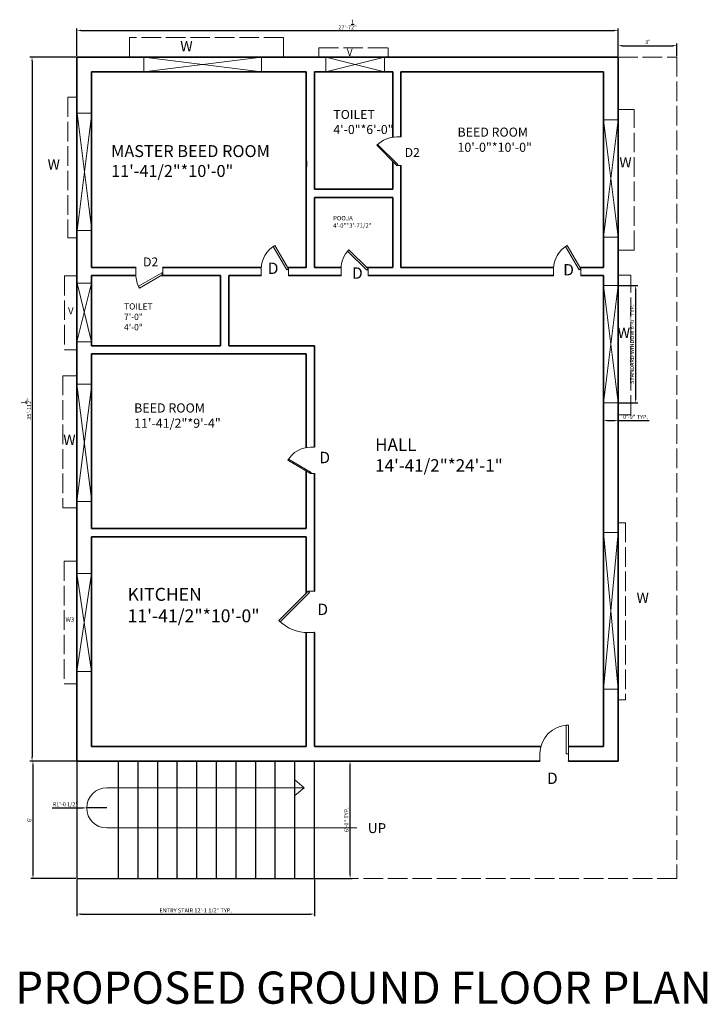
# Model space of a CAD drawing. Units: millimetres. Extents: x 3312 to 4717, y 967 to 1587.
# Tile 1 of 2: x 3312 to 3733, y 967 to 1571. Entities that reach past the tile are written whole.
import ezdxf

# ---------------------------------------------------------------- set-up
doc = ezdxf.new("R2010")
doc.units = ezdxf.units.MM
doc.linetypes.add('ACAD_ISO02W100', pattern=[15, 12, -3])
for name, color, linetype, lineweight, true_color in [('A-ANNO-DIMS', 116, 'Continuous', 18, 0x136734), ('A-ANNO-IDEN', 116, 'Continuous', 18, 0x136734), ('A-ANNO-SYMB', 219, 'Continuous', 18, 0x642165), ('A-ANNO-TEXT', 55, 'Continuous', 18, 0x999b37), ('A-ANNO-TITL', 116, 'Continuous', 35, 0x136734), ('A-AREA-IDEN', 244, 'Continuous', 18, 0x991b1e), ('A-GLAZ', 219, 'Continuous', 18, 0x642165), ('A-GLAZ-OVHD', 67, 'ACAD_ISO02W100', 13, 0x727430), ('C-PROP', 67, 'ACAD_ISO02W100', 18, 0x727430)]:
    doc.layers.add(name, color=color, linetype=linetype, lineweight=lineweight, true_color=true_color)
for name, color, linetype, lineweight in [('A-DOOR', 4, 'Continuous', 18), ('A-FLOR-STRS', 7, 'Continuous', 25), ('A-WALL', 7, 'Continuous', 35)]:
    doc.layers.add(name, color=color, linetype=linetype, lineweight=lineweight)
doc.styles.get("Standard").update_dxf_attribs({"font": 'arial.ttf'})
doc.dimstyles.new('ISO-25', dxfattribs={"dimtxt": 2.5, "dimasz": 2.5, "dimexe": 1.25, "dimexo": 0.625, "dimtad": 1, "dimdec": 3, "dimlunit": 4, "dimtxsty": 'Standard', "dimcen": 2.5, "dimadec": 0, "dimazin": 0, "dimtfac": 1, "dimtdec": 3, "dimtmove": 0, "dimatfit": 3, "dimfxl": 1, "dimarcsym": 0})

# ---------------------------------------------------------------- blocks, each defined once
blk = doc.blocks.new('*U3')
for p, q in [((-24, 0), (-24, 6)), ((0, 0), (0, 6))]:
    blk.add_line(p, q)
blk.add_lwpolyline([(0, 0), (-20.78, -12), (-21.66, -10.48), (-0.88, 1.52)], close=True)
blk.add_arc((0, 0), 24, 180, 210)
blk = doc.blocks.new('*U4')
for p, q in [((-24, 0), (-24, -6)), ((0, 0), (0, -6))]:
    blk.add_line(p, q)
blk.add_lwpolyline([(0, 0), (-12, 20.78), (-13.52, 19.91), (-1.52, -0.88)], close=True)
blk.add_arc((0, 0), 24, 120, 180)
blk = doc.blocks.new('*U5')
for p, q in [((0, 0), (0, -6)), ((40, 0), (40, -6))]:
    blk.add_line(p, q)
blk.add_lwpolyline([(0, 0), (28.3, 28.3), (29.5, 27), (1.2, -1.2)], close=True)
blk.add_arc((0, 0), 40, 0, 45)
blk = doc.blocks.new('*U7')
for p, q in [((0, 0), (0, -6)), ((40, 0), (40, -6))]:
    blk.add_line(p, q)
blk.add_lwpolyline([(0, 0), (20, 34.6), (21.5, 33.8), (1.5, -0.9)], close=True)
blk.add_arc((0, 0), 40, 0, 60)
blk = doc.blocks.new('*U6')
for p, q in [((0, 0), (0, 6)), ((40, 0), (40, 6))]:
    blk.add_line(p, q)
blk.add_lwpolyline([(0, 0), (28.28, -28.28), (29.52, -27.05), (1.24, 1.24)], close=True)
blk.add_arc((0, 0), 40, 315, 360)
blk = doc.blocks.new('*U2')
for p, q in [((0, 0), (0, -6)), ((24, 0), (24, -6))]:
    blk.add_line(p, q)
blk.add_lwpolyline([(0, 0), (0, 24), (1.75, 24), (1.75, 0)], close=True)
blk.add_arc((0, 0), 24, 0, 90)
blk = doc.blocks.new('*U8')
for p, q in [((-24, 0), (-24, -6)), ((0, 0), (0, -6))]:
    blk.add_line(p, q)
blk.add_lwpolyline([(0, 0), (-16.97, 16.97), (-18.21, 15.73), (-1.24, -1.24)], close=True)
blk.add_arc((0, 0), 24, 135, 180)
blk = doc.blocks.new('*D9')
at = {"layer": 'A-ANNO-DIMS', "color": 0, "lineweight": -2, "transparency": 16777216}
for p, q in [((3678.84, 1548.26), (3678.84, 1555.85)), ((3681.34, 1554.6), (3712.34, 1554.6)), ((3714.84, 1548.26), (3714.84, 1555.85))]:
    blk.add_line(p, q, dxfattribs=at)
at = {"layer": 'A-ANNO-DIMS', "color": 0, "lineweight": 5, "transparency": 16777216}
for points in [[(3681.34, 1555.02), (3681.34, 1554.18), (3678.84, 1554.6)], [(3712.34, 1555.02), (3712.34, 1554.18), (3714.84, 1554.6)]]:
    blk.add_solid(points, dxfattribs=at)
at = {"layer": 'Defpoints', "color": 0, "lineweight": 5, "transparency": 16777216}
for p in [(3714.84, 1554.6), (3678.84, 1547.64), (3714.84, 1547.64)]:
    blk.add_point(p, dxfattribs=at)
at = {"layer": 'A-ANNO-DIMS', "color": 0, "transparency": 16777216, "insert": (3696.84, 1556.5), "char_height": 2.5, "attachment_point": 5}
blk.add_mtext("3'", dxfattribs=at)
blk = doc.blocks.new('*D10')
at = {"layer": 'A-ANNO-DIMS', "color": 0, "lineweight": -2, "transparency": 16777216}
for p, q in [((3347.34, 1548.26), (3347.34, 1565.23)), ((3349.84, 1563.98), (3676.34, 1563.98)), ((3678.84, 1548.26), (3678.84, 1565.23))]:
    blk.add_line(p, q, dxfattribs=at)
at = {"layer": 'A-ANNO-DIMS', "color": 0, "lineweight": 5, "transparency": 16777216}
for points in [[(3349.84, 1564.4), (3349.84, 1563.57), (3347.34, 1563.98)], [(3676.34, 1564.4), (3676.34, 1563.57), (3678.84, 1563.98)]]:
    blk.add_solid(points, dxfattribs=at)
at = {"layer": 'Defpoints', "color": 0, "lineweight": 5, "transparency": 16777216}
for p in [(3678.84, 1563.98), (3347.34, 1547.64), (3678.84, 1547.64)]:
    blk.add_point(p, dxfattribs=at)
at = {"layer": 'A-ANNO-DIMS', "color": 0, "transparency": 16777216, "insert": (3513.09, 1567.54), "char_height": 2.5, "attachment_point": 5}
blk.add_mtext('27\'-7{\\H1x;\\S1/2;}"', dxfattribs=at)
blk = doc.blocks.new('*D11')
at = {"layer": 'A-ANNO-DIMS', "color": 0, "lineweight": -2, "transparency": 16777216}
for p, q in [((3346.71, 1547.64), (3318.6, 1547.64)), ((3319.85, 1545.14), (3319.85, 1118.64)), ((3346.71, 1116.14), (3318.6, 1116.14))]:
    blk.add_line(p, q, dxfattribs=at)
at = {"layer": 'A-ANNO-DIMS', "color": 0, "lineweight": 5, "transparency": 16777216}
for points in [[(3319.43, 1545.14), (3320.27, 1545.14), (3319.85, 1547.64)], [(3319.43, 1118.64), (3320.27, 1118.64), (3319.85, 1116.14)]]:
    blk.add_solid(points, dxfattribs=at)
at = {"layer": 'Defpoints', "color": 0, "lineweight": 5, "transparency": 16777216}
for p in [(3347.34, 1547.64), (3319.85, 1116.14), (3347.34, 1116.14)]:
    blk.add_point(p, dxfattribs=at)
at = {"layer": 'A-ANNO-DIMS', "color": 0, "transparency": 16777216, "insert": (3316.27, 1331.89), "char_height": 2.5, "attachment_point": 5, "rotation": 90}
blk.add_mtext('35\'-11{\\H1x;\\S1/2;}"', dxfattribs=at)
blk = doc.blocks.new('*D12')
at = {"layer": 'A-ANNO-DIMS', "color": 0, "lineweight": -2, "transparency": 16777216}
for p, q in [((3346.71, 1116.14), (3319.16, 1116.14)), ((3320.41, 1113.64), (3320.41, 1046.64)), ((3346.71, 1044.14), (3319.16, 1044.14))]:
    blk.add_line(p, q, dxfattribs=at)
at = {"layer": 'A-ANNO-DIMS', "color": 0, "lineweight": 5, "transparency": 16777216}
for points in [[(3320, 1113.64), (3320.83, 1113.64), (3320.41, 1116.14)], [(3320, 1046.64), (3320.83, 1046.64), (3320.41, 1044.14)]]:
    blk.add_solid(points, dxfattribs=at)
at = {"layer": 'Defpoints', "color": 0, "lineweight": 5, "transparency": 16777216}
for p in [(3347.34, 1116.14), (3320.41, 1044.14), (3347.34, 1044.14)]:
    blk.add_point(p, dxfattribs=at)
at = {"layer": 'A-ANNO-DIMS', "color": 0, "transparency": 16777216, "insert": (3318.51, 1080.14), "char_height": 2.5, "attachment_point": 5, "rotation": 90}
blk.add_mtext("6'", dxfattribs=at)
blk = doc.blocks.new('WIN-STANDARD')
for p, q in [((0, 72), (0, 0)), ((0, 0), (9, 72)), ((9, 72), (0, 72)), ((0, 72), (9, 0)), ((9, 0), (9, 72)), ((0, 0), (9, 0)), ((9, 0), (0, 0))]:
    blk.add_line(p, q)
blk = doc.blocks.new('GLAZ-NARROW')
for p, q in [((9, 35.99), (0.01, 35.99)), ((0.01, 35.99), (0.01, 0)), ((0.01, 0), (9, 35.99)), ((0.07, 35.99), (9, 0)), ((9, 0), (9, 35.99)), ((0, 0), (9, 0))]:
    blk.add_line(p, q)
blk = doc.blocks.new('STAIR-ENTRY-FLIGHT')
for p, q in [((0, 72), (0, 0)), ((145.5, 72), (0, 72)), ((25.5, 0), (25.5, 72)), ((37.5, 0), (37.5, 72)), ((49.5, 0), (49.5, 72)), ((61.5, 0), (61.5, 72)), ((73.5, 0), (73.5, 72)), ((85.5, 0), (85.5, 72)), ((97.5, 0), (97.5, 72)), ((109.5, 0), (109.5, 72)), ((121.5, 0), (121.5, 72)), ((133.5, 0), (133.5, 72)), ((145.5, 0), (145.5, 72)), ((0, 0), (145.5, 0))]:
    blk.add_line(p, q)
blk = doc.blocks.new('*D26')
at = {"layer": 'A-ANNO-DIMS', "color": 0, "lineweight": -2, "transparency": 16777216}
for p, q in [((3679.46, 1407.62), (3690.89, 1407.62)), ((3689.64, 1338.12), (3689.64, 1405.12)), ((3679.46, 1335.62), (3690.89, 1335.62))]:
    blk.add_line(p, q, dxfattribs=at)
at = {"layer": 'A-ANNO-DIMS', "color": 0, "lineweight": 5, "transparency": 16777216}
for points in [[(3689.22, 1405.12), (3690.05, 1405.12), (3689.64, 1407.62)], [(3689.22, 1338.12), (3690.05, 1338.12), (3689.64, 1335.62)]]:
    blk.add_solid(points, dxfattribs=at)
at = {"layer": 'Defpoints', "color": 0, "lineweight": 5, "transparency": 16777216}
for p in [(3678.84, 1407.62), (3689.64, 1407.62), (3678.84, 1335.62)]:
    blk.add_point(p, dxfattribs=at)
at = {"layer": 'A-ANNO-DIMS', "color": 0, "transparency": 16777216, "insert": (3687.72, 1371.62), "char_height": 2.5, "attachment_point": 5, "rotation": 90}
blk.add_mtext('STANDARD WINDOW 6\'-0" TYP.', dxfattribs=at)
blk = doc.blocks.new('*D27')
at = {"layer": 'A-ANNO-DIMS', "color": 0, "lineweight": -2, "transparency": 16777216}
for p, q in [((3669.84, 1335), (3669.84, 1323.57)), ((3678.84, 1335), (3678.84, 1323.57)), ((3672.34, 1324.82), (3676.34, 1324.82)), ((3678.84, 1324.82), (3697.82, 1324.82))]:
    blk.add_line(p, q, dxfattribs=at)
at = {"layer": 'A-ANNO-DIMS', "color": 0, "lineweight": 5, "transparency": 16777216}
for points in [[(3672.34, 1325.24), (3672.34, 1324.4), (3669.84, 1324.82)], [(3676.34, 1325.24), (3676.34, 1324.4), (3678.84, 1324.82)]]:
    blk.add_solid(points, dxfattribs=at)
at = {"layer": 'Defpoints', "color": 0, "lineweight": 5, "transparency": 16777216}
for p in [(3669.84, 1335.62), (3678.84, 1335.62), (3678.84, 1324.82)]:
    blk.add_point(p, dxfattribs=at)
at = {"layer": 'A-ANNO-DIMS', "color": 0, "transparency": 16777216, "insert": (3689.58, 1326.72), "char_height": 2.5, "attachment_point": 5}
blk.add_mtext('0\'-9" TYP.', dxfattribs=at)
blk = doc.blocks.new('*D32')
at = {"layer": 'A-ANNO-DIMS', "color": 0, "lineweight": -2, "transparency": 16777216}
for p, q in [((3347.34, 1043.51), (3347.34, 1021.06)), ((3492.84, 1043.51), (3492.84, 1021.06)), ((3349.84, 1022.31), (3490.34, 1022.31))]:
    blk.add_line(p, q, dxfattribs=at)
at = {"layer": 'A-ANNO-DIMS', "color": 0, "lineweight": 5, "transparency": 16777216}
for points in [[(3349.84, 1022.73), (3349.84, 1021.9), (3347.34, 1022.31)], [(3490.34, 1022.73), (3490.34, 1021.9), (3492.84, 1022.31)]]:
    blk.add_solid(points, dxfattribs=at)
at = {"layer": 'Defpoints', "color": 0, "lineweight": 5, "transparency": 16777216}
for p in [(3347.34, 1044.14), (3492.84, 1044.14), (3492.84, 1022.31)]:
    blk.add_point(p, dxfattribs=at)
at = {"layer": 'A-ANNO-DIMS', "color": 0, "transparency": 16777216, "insert": (3420.09, 1024.23), "char_height": 2.5, "attachment_point": 5}
blk.add_mtext('ENTRY STAIR 12\'-1 1/2" TYP.', dxfattribs=at)
blk = doc.blocks.new('*D33')
at = {"layer": 'A-ANNO-DIMS', "color": 0, "lineweight": -2, "transparency": 16777216}
for p, q in [((3493.46, 1116.14), (3515.91, 1116.14)), ((3514.66, 1046.64), (3514.66, 1113.64)), ((3493.46, 1044.14), (3515.91, 1044.14))]:
    blk.add_line(p, q, dxfattribs=at)
at = {"layer": 'A-ANNO-DIMS', "color": 0, "lineweight": 5, "transparency": 16777216}
for points in [[(3514.25, 1113.64), (3515.08, 1113.64), (3514.66, 1116.14)], [(3514.25, 1046.64), (3515.08, 1046.64), (3514.66, 1044.14)]]:
    blk.add_solid(points, dxfattribs=at)
at = {"layer": 'Defpoints', "color": 0, "lineweight": 5, "transparency": 16777216}
for p in [(3492.84, 1116.14), (3514.66, 1116.14), (3492.84, 1044.14)]:
    blk.add_point(p, dxfattribs=at)
at = {"layer": 'A-ANNO-DIMS', "color": 0, "transparency": 16777216, "insert": (3512.76, 1080.14), "char_height": 2.5, "attachment_point": 5, "rotation": 90}
blk.add_mtext('6\'-0" TYP.', dxfattribs=at)
blk = doc.blocks.new('*D38')
at = {"layer": 'A-ANNO-DIMS', "color": 0, "lineweight": -2, "transparency": 16777216}
for p, q in [((3332.21, 1087.39), (3350.83, 1087.39)), ((3365.62, 1087.39), (3353.33, 1087.39))]:
    blk.add_line(p, q, dxfattribs=at)
at = {"layer": 'A-ANNO-DIMS', "color": 0, "lineweight": 5, "transparency": 16777216}
blk.add_solid([(3350.83, 1087.81), (3350.83, 1086.98), (3353.33, 1087.39)], dxfattribs=at)
at = {"layer": 'Defpoints', "color": 0, "lineweight": 5, "transparency": 16777216}
for p in [(3353.33, 1087.39), (3365.62, 1087.39)]:
    blk.add_point(p, dxfattribs=at)
at = {"layer": 'A-ANNO-DIMS', "color": 0, "transparency": 16777216, "insert": (3340.27, 1089.31), "char_height": 2.5, "attachment_point": 5, "rotation": 359.9993}
blk.add_mtext('R1\'-0 1/2"', dxfattribs=at)

msp = doc.modelspace()

# ---------------------------------------------------------------- linework, layer by layer
at = {"layer": 'A-ANNO-SYMB'}
for p, q in [((3486.4542, 1099.6819), (3480.8387, 1104.6174)), ((3480.8387, 1104.6174), (3480.8387, 1094.9798)), ((3365.6152, 1099.6819), (3486.4542, 1099.6819)), ((3486.4542, 1099.6819), (3480.8387, 1094.9798)), ((3480.8387, 1094.9798), (3486.4542, 1099.6819)), ((3518.8463, 1075.1058), (3365.6152, 1075.1058)), ((3372.8387, 1075.1058), (3518.8463, 1075.1058))]:
    msp.add_line(p, q, dxfattribs=at)
msp.add_arc((3365.6152, 1087.3938), 12.2881, 90, 270, dxfattribs=at)
at = {"layer": 'A-GLAZ'}
for p, q in [((3388.349, 1547.6367), (3388.349, 1538.6367)), ((3460.349, 1547.6367), (3388.349, 1547.6367)), ((3388.349, 1547.6367), (3460.349, 1538.6367)), ((3460.349, 1547.6367), (3388.349, 1538.6367)), ((3388.349, 1538.6367), (3388.349, 1547.6367)), ((3460.349, 1538.6367), (3460.349, 1547.6367)), ((3460.349, 1538.6367), (3460.349, 1547.6367)), ((3499.8135, 1547.6367), (3499.8135, 1538.6367)), ((3535.813, 1547.6367), (3499.8135, 1547.6367)), ((3535.813, 1547.6367), (3499.8135, 1538.6367)), ((3499.8135, 1538.6367), (3499.8135, 1547.6367)), ((3499.8135, 1547.6367), (3535.813, 1538.6367)), ((3535.813, 1538.4566), (3535.813, 1547.6367)), ((3535.813, 1538.4566), (3535.813, 1547.6367)), ((3388.349, 1538.6367), (3460.349, 1538.6367)), ((3499.8135, 1538.6367), (3535.813, 1538.6367)), ((3669.8387, 1160.1744), (3669.8387, 1256.1744)), ((3669.8387, 1256.1744), (3669.8387, 1256.1744)), ((3669.8387, 1256.1744), (3678.8387, 1256.1744)), ((3678.8387, 1160.1744), (3669.8387, 1256.1744)), ((3669.8387, 1256.1744), (3678.8387, 1256.1744)), ((3678.8387, 1256.1744), (3669.8387, 1160.1744)), ((3678.8387, 1256.1744), (3678.8387, 1160.1744)), ((3356.3387, 1231.0262), (3347.3387, 1231.0262)), ((3347.3387, 1231.0262), (3347.3387, 1171.0262)), ((3356.3387, 1231.0262), (3347.3387, 1171.0262)), ((3356.3387, 1171.0262), (3347.3387, 1231.0262)), ((3356.3387, 1171.0262), (3356.3387, 1231.0262)), ((3347.3387, 1171.0262), (3356.3387, 1171.0262)), ((3347.3387, 1171.0262), (3356.3387, 1171.0262)), ((3678.8387, 1160.1744), (3669.8387, 1160.1744))]:
    msp.add_line(p, q, dxfattribs=at)
at = {"layer": 'A-GLAZ-OVHD'}
for p, q in [((3473.8562, 1559.646), (3379.4749, 1559.646)), ((3379.4749, 1559.646), (3379.4749, 1547.6367)), ((3473.8562, 1547.6367), (3473.8562, 1559.646)), ((3495.5448, 1547.6367), (3495.5448, 1553.3254)), ((3495.5448, 1553.3254), (3537.9357, 1553.3254)), ((3537.9357, 1553.3254), (3537.9357, 1547.6367)), ((3347.3387, 1522.9718), (3341.7625, 1522.9718)), ((3341.7625, 1522.9718), (3341.7625, 1436.8594)), ((3688.7267, 1515.5849), (3678.8387, 1515.5849)), ((3688.7267, 1429.2679), (3688.7267, 1515.5849)), ((3341.7625, 1436.8594), (3347.3387, 1436.8594)), ((3678.8387, 1429.2679), (3688.7267, 1429.2679)), ((3347.3387, 1413.4775), (3339.7577, 1413.4775)), ((3339.7577, 1413.4775), (3339.7577, 1368.2136)), ((3686.5629, 1413.9949), (3678.8387, 1413.9949)), ((3686.5629, 1328.3259), (3686.5629, 1413.9949)), ((3339.7577, 1368.2136), (3347.3387, 1368.2136)), ((3347.3387, 1352.3145), (3338.7442, 1352.3145)), ((3338.7442, 1352.3145), (3338.7442, 1271.2968)), ((3678.8387, 1328.3259), (3686.5629, 1328.3259)), ((3338.7442, 1271.2968), (3347.3387, 1271.2968)), ((3678.8387, 1262.2292), (3683.4637, 1262.2292)), ((3683.4637, 1262.2292), (3683.4637, 1153.655)), ((3347.3387, 1238.5495), (3339.4532, 1238.5495)), ((3339.4532, 1238.5495), (3339.4532, 1163.5136)), ((3339.4532, 1163.5136), (3347.3387, 1163.5136)), ((3683.4637, 1153.655), (3678.8387, 1153.655))]:
    msp.add_line(p, q, dxfattribs=at)
at = {"layer": 'A-WALL'}
for p, q in [((3347.3387, 1547.6367), (3678.8387, 1547.6367)), ((3347.3387, 1116.1367), (3347.3387, 1547.6367)), ((3678.8387, 1547.6367), (3678.8387, 1116.1367)), ((3356.3387, 1538.6367), (3487.8387, 1538.6367)), ((3356.3387, 1418.6367), (3356.3387, 1538.6367)), ((3487.8387, 1476.3517), (3487.8387, 1538.6367)), ((3492.8387, 1538.6367), (3540.8387, 1538.6367)), ((3492.8387, 1466.6367), (3492.8387, 1538.6367)), ((3540.8387, 1498.4759), (3540.8387, 1538.6367)), ((3545.8387, 1538.6367), (3669.8387, 1538.6367)), ((3545.8387, 1498.6511), (3545.8387, 1538.6367)), ((3669.8387, 1538.6367), (3669.8387, 1418.6367)), ((3487.8387, 1476.3517), (3487.8853, 1484.1241)), ((3492.8387, 1475.4852), (3492.8387, 1480.9263)), ((3540.8387, 1466.6367), (3540.8387, 1483.6633)), ((3545.8387, 1418.6367), (3545.8387, 1481.1963)), ((3487.8387, 1418.6367), (3487.8387, 1476.3517)), ((3492.8387, 1466.6367), (3492.8387, 1475.4852)), ((3492.8387, 1466.6367), (3540.8387, 1466.6367)), ((3492.8387, 1461.6367), (3540.8387, 1461.6367)), ((3492.8387, 1418.6367), (3492.8387, 1461.6367)), ((3540.8387, 1418.6367), (3540.8387, 1461.6367)), ((3356.3387, 1418.6367), (3382.6748, 1418.6367)), ((3382.6748, 1418.6367), (3383.4216, 1418.6367)), ((3383.4216, 1418.6367), (3383.4216, 1418.5704)), ((3383.4216, 1418.6271), (3383.4216, 1418.5137)), ((3400.0402, 1418.6367), (3435.3387, 1418.6367)), ((3400.0402, 1418.5137), (3400.0402, 1418.6367)), ((3435.3387, 1418.6367), (3460.1074, 1418.6367)), ((3460.1074, 1418.6367), (3460.3086, 1418.6369)), ((3476.4113, 1418.6367), (3487.8387, 1418.6367)), ((3492.8387, 1418.6367), (3509.1468, 1418.6367)), ((3524.888, 1418.6367), (3540.8387, 1418.6367)), ((3545.8387, 1418.6367), (3639.3589, 1418.6367)), ((3655.4616, 1418.6367), (3669.8387, 1418.6367)), ((3356.3387, 1413.6367), (3383.4373, 1413.6367)), ((3356.3387, 1370.6367), (3356.3387, 1413.6367)), ((3398.7891, 1413.6367), (3435.3387, 1413.6367)), ((3435.3387, 1370.6367), (3435.3387, 1413.6367)), ((3440.3387, 1370.6367), (3440.3387, 1413.6367)), ((3440.3387, 1413.6367), (3459.637, 1413.6367)), ((3459.637, 1413.6367), (3460.2866, 1413.6367)), ((3476.9052, 1413.6367), (3509.1248, 1413.6367)), ((3525.7434, 1413.6367), (3639.3589, 1413.6367)), ((3655.9728, 1413.6367), (3655.9555, 1413.7668)), ((3655.9555, 1413.6367), (3669.8387, 1413.6367)), ((3669.8387, 1413.6367), (3669.8387, 1352.8861)), ((3356.3387, 1370.6367), (3435.3387, 1370.6367)), ((3440.3387, 1370.6367), (3492.8387, 1370.6367)), ((3492.8387, 1370.6367), (3492.8387, 1365.6367)), ((3356.3387, 1365.6367), (3487.8387, 1365.6367)), ((3356.3387, 1258.6367), (3356.3387, 1365.6367)), ((3487.8387, 1365.6367), (3487.8387, 1308.2785)), ((3487.8387, 1308.2785), (3487.8387, 1365.6367)), ((3492.8387, 1308.4934), (3492.8387, 1365.6367)), ((3669.8387, 1365.6367), (3669.8387, 1125.1367)), ((3487.8387, 1258.6367), (3487.8387, 1293.9359)), ((3487.8387, 1293.9359), (3487.8387, 1258.6367)), ((3492.8387, 1220.1962), (3492.8387, 1292.424)), ((3487.8387, 1258.6367), (3356.3387, 1258.6367)), ((3356.3387, 1125.1367), (3356.3387, 1253.6367)), ((3487.8387, 1253.6367), (3356.3387, 1253.6367)), ((3487.8387, 1253.6367), (3487.8387, 1253.6367)), ((3487.8387, 1219.0672), (3487.8387, 1253.6367)), ((3492.7695, 1220.1962), (3492.8387, 1220.1962)), ((3487.8387, 1125.1367), (3487.8387, 1194.8755)), ((3492.8387, 1194.8397), (3492.7695, 1194.8503)), ((3492.8387, 1125.1367), (3492.8387, 1194.8397)), ((3487.8387, 1125.1367), (3356.3387, 1125.1367)), ((3631.5285, 1125.1367), (3492.8387, 1125.1367)), ((3669.8387, 1125.1367), (3648.385, 1125.1367)), ((3630.9238, 1116.1367), (3347.3387, 1116.1367)), ((3630.9238, 1116.2159), (3630.9238, 1116.1367)), ((3648.3974, 1116.1367), (3648.385, 1116.2159)), ((3678.8387, 1116.1367), (3648.3974, 1116.1367))]:
    msp.add_line(p, q, dxfattribs=at)
at = {"layer": 'C-PROP'}
for p, q in [((3678.8387, 1547.6367), (3714.8387, 1547.6367)), ((3714.8387, 1547.6367), (3714.8387, 1044.1367)), ((3714.8387, 1044.1367), (3492.8387, 1044.1367))]:
    msp.add_line(p, q, dxfattribs=at)

# ---------------------------------------------------------------- block references
at = {"layer": 'A-DOOR'}
for name, p, xscale, yscale, zscale, rotation in [('*U5', (3543.3057, 1481.1963), 0.436369325582765, 0.436369325582765, 0.436369325582765, 90), ('*U7', (3490.4575, 1292.424), 0.4017342436988492, 0.4017342436988492, 0.4017342436988492, 90), ('*U6', (3488.9677, 1220.1962), 0.6336462587443874, 0.6336462587443874, 0.6336462587443874, 270)]:
    msp.add_blockref(name, p, dxfattribs=dict(at, xscale=xscale, yscale=yscale, zscale=zscale, rotation=rotation))
for name, p, xscale, yscale, zscale in [('*U4', (3476.9052, 1417.7814), 0.6924402839390947, 0.6924402839390947, 0.6924402839390947), ('*U4', (3655.9555, 1417.7814), 0.6924402839390947, 0.6924402839390947, 0.6924402839390947), ('*U8', (3525.7434, 1417.7814), 0.6924402839390947, 0.6924402839390947, 0.6924402839390947), ('*U3', (3400.0402, 1414.3591), 0.6924402839390947, 0.6924402839390947, 0.6924402839390947), ('*U2', (3648.385, 1120.5812), -0.7275510770565516, 0.7275510770565516, 0.7275510770565516)]:
    msp.add_blockref(name, p, dxfattribs=dict(at, xscale=xscale, yscale=yscale, zscale=zscale))
at = {"layer": 'A-FLOR-STRS'}
msp.add_blockref('STAIR-ENTRY-FLIGHT', (3347.339, 1044.137), dxfattribs=at)
at = {"layer": 'A-GLAZ'}
for name, p in [('WIN-STANDARD', (3347.4465, 1441.2557)), ('WIN-STANDARD', (3669.8935, 1437.2023)), ('GLAZ-NARROW', (3347.339, 1373.056)), ('WIN-STANDARD', (3669.8357, 1335.6213)), ('WIN-STANDARD', (3347.38, 1275.137))]:
    msp.add_blockref(name, p, dxfattribs=at)

# ---------------------------------------------------------------- texts
at = {"layer": 'A-ANNO-IDEN', "attachment_point": 1}
for s, width, gutter_width, insert, char_height in [('W', 58.784208, 31.4406, (3410.6717, 1557.4065), 6.2881), ('V', 17.492344, 22.1494, (3512.7061, 1552.7106), 4.4299), ('D2', 38.407199, 27.2994, (3548.1385, 1491.8809), 5.45989), ('W', 58.784208, 31.4406, (3329.3879, 1484.9586), 6.2881), ('W', 58.784208, 31.4406, (3679.6139, 1486.258), 6.2881), ('D2', 38.407199, 27.2994, (3387.886, 1424.7858), 5.45989), ('D', 165.385008, 34.9095, (3464.2354, 1421.6504), 6.9819), ('D', 165.385008, 34.9095, (3515.8541, 1418.7208), 6.9819), ('D', 165.385008, 34.9095, (3645.24, 1420.7551), 6.9819), ('V', 17.492344, 22.1494, (3341.841, 1394.304), 4.4299), ('W', 58.784208, 31.4406, (3678.6366, 1381.7766), 6.2881), ('W', 58.784208, 31.4406, (3339.001, 1316.202), 6.2881), ('D', 165.385008, 34.9095, (3495.8618, 1305.6662), 6.9819), ('W', 58.784208, 31.4406, (3690.1575, 1219.3404), 6.2881), ('D', 165.385008, 34.9095, (3494.6584, 1212.5975), 6.9819), ('W3', 5.651424, 13.549, (3340.3545, 1204.2197), 2.7098), ('D', 165.385008, 34.9095, (3635.2944, 1109.0258), 6.9819)]:
    msp.add_mtext_dynamic_manual_height_columns(s, width=width, gutter_width=gutter_width, heights=[0], dxfattribs=dict(at, insert=insert, char_height=char_height))
at = {"layer": 'A-ANNO-TEXT', "insert": (3525.5354, 1078.0463), "char_height": 6.06981, "attachment_point": 1}
msp.add_mtext_dynamic_manual_height_columns('UP', width=66.331887, gutter_width=30.349, heights=[0], dxfattribs=at)
at = {"layer": 'A-ANNO-TITL', "insert": (3309.5799, 987.0951), "char_height": 19.730766, "attachment_point": 1}
msp.add_mtext_dynamic_manual_height_columns('PROPOSED GROUND FLOOR PLAN', width=589.074298, gutter_width=98.6538, heights=[0], dxfattribs=at)
at = {"layer": 'A-AREA-IDEN', "attachment_point": 1}
for s, width, gutter_width, insert, char_height in [('TOILET\\P4\'-0"*6\'-0"', 186.434458, 27.6289, (3504.4296, 1515.1946), 5.525778), ('BEED ROOM\\P10\'-0"*10\'-0"', 233.542976, 27.8672, (3580.4729, 1504.4089), 5.573446), ('MASTER BEED ROOM\\P11\'-41/2"*10\'-0"', 255.898299, 36.5736, (3368.302, 1493.653), 7.31472), ('POOJA\\P4\'-0"*3\'-71/2"', 27.191905, 13.5214, (3504.2633, 1450.222), 2.704284), ('TOILET\\P7\'-0"\\P4\'-0"', 71.714913, 19.0789, (3376.2077, 1396.6906), 3.81577), ('BEED ROOM\\P11\'-41/2"*9\'-4"', 153.649849, 28.0299, (3382.3697, 1335.3464), 5.605977), ('HALL\\P14\'-41/2"*24\'-1"', 355.259397, 38.2085, (3530.0231, 1313.878), 7.641696), ('KITCHEN\\P11\'-41/2"*10\'-0"', 221.328825, 39.5346, (3378.3702, 1222.2691), 7.906913)]:
    msp.add_mtext_dynamic_manual_height_columns(s, width=width, gutter_width=gutter_width, heights=[0], dxfattribs=dict(at, insert=insert, char_height=char_height))

# ---------------------------------------------------------------- dimensions: what is measured, and where the dimension line sits
at = {"layer": 'A-ANNO-DIMS'}
for base, p1, p2, picture, middle in [((3678.8387, 1563.9847), (3347.3387, 1547.6367), (3678.8387, 1547.6367), '*D10', (3513.0887, 1567.5366)), ((3714.8387, 1554.5984), (3678.8387, 1547.6367), (3714.8387, 1547.6367), '*D9', (3696.8387, 1556.5007))]:
    dim = msp.add_linear_dim(base=base, p1=p1, p2=p2, dimstyle='ISO-25', override={"dimclrd": 0, "dimclre": 0, "dimclrt": 0}, dxfattribs=at)
    dim.commit()
    dim.dimension.update_dxf_attribs({"geometry": picture, "text_midpoint": middle})
for base, p1, p2, picture, middle in [((3319.8488, 1116.1367), (3347.3387, 1547.6367), (3347.3387, 1116.1367), '*D11', (3316.2748, 1331.8867)), ((3320.413, 1044.1367), (3347.3387, 1116.1367), (3347.3387, 1044.1367), '*D12', (3318.5116, 1080.1367))]:
    dim = msp.add_linear_dim(base=base, p1=p1, p2=p2, angle=90, dimstyle='ISO-25', override={"dimclrd": 0, "dimclre": 0, "dimclrt": 0}, dxfattribs=at)
    dim.commit()
    dim.dimension.update_dxf_attribs({"geometry": picture, "text_midpoint": middle})
for base, p1, p2, text, picture, middle in [((3689.6362, 1407.6217), (3678.8362, 1335.6217), (3678.8362, 1407.6217), 'STANDARD WINDOW <> TYP.', '*D26', (3687.7177, 1371.6217)), ((3514.6637, 1116.1367), (3492.8387, 1044.1367), (3492.8387, 1116.1367), '<> TYP.', '*D33', (3512.7623, 1080.1367))]:
    dim = msp.add_linear_dim(base=base, p1=p1, p2=p2, angle=90, text=text, dimstyle='ISO-25', override={"dimdec": 1, "dimlfac": 1, "dimrnd": 0, "dimzin": 1, "dimdsep": 46, "dimlunit": 4, "dimfrac": 2}, dxfattribs=at)
    dim.commit()
    dim.dimension.update_dxf_attribs({"geometry": picture, "text_midpoint": middle})
for base, p1, p2, text, picture, middle in [((3678.8362, 1324.8217), (3669.8362, 1335.6217), (3678.8362, 1335.6217), '<> TYP.', '*D27', (3689.5805, 1326.7231)), ((3492.8387, 1022.3117), (3347.3387, 1044.1367), (3492.8387, 1044.1367), 'ENTRY STAIR <> TYP.', '*D32', (3420.0887, 1024.2294))]:
    dim = msp.add_linear_dim(base=base, p1=p1, p2=p2, text=text, dimstyle='ISO-25', override={"dimdec": 1, "dimlfac": 1, "dimrnd": 0, "dimzin": 1, "dimdsep": 46, "dimlunit": 4, "dimfrac": 2}, dxfattribs=at)
    dim.commit()
    dim.dimension.update_dxf_attribs({"geometry": picture, "text_midpoint": middle})
dim = msp.add_radius_dim(center=(3365.6152, 1087.3938), mpoint=(3353.3271, 1087.394), dimstyle='ISO-25', override={"dimdec": 1, "dimlfac": 1, "dimrnd": 0, "dimzin": 1, "dimdsep": 46, "dimlunit": 4, "dimfrac": 2}, dxfattribs=at)
dim.commit()
dim.dimension.update_dxf_attribs({"geometry": '*D38', "text_midpoint": (3340.2703, 1089.3118)})

doc.saveas('drawing.dxf')
